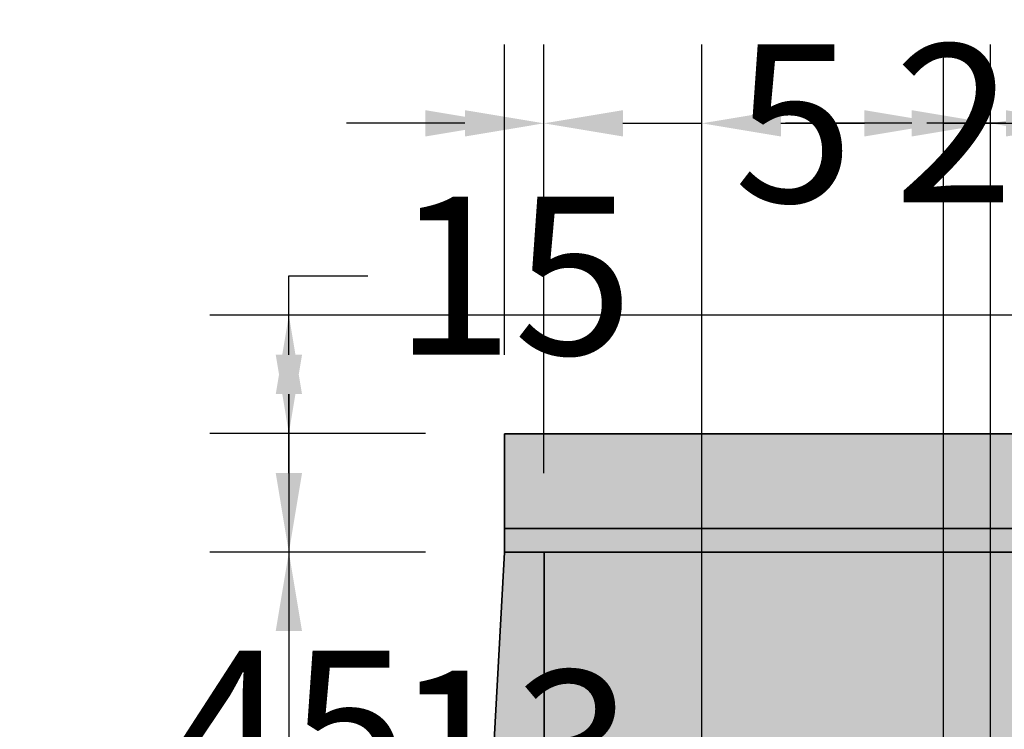
# Model space of a CAD drawing. Units: millimetres. Extents: x 130 to 1021, y 147 to 699.
# Tile 18 of 40: x 241 to 366, y 610 to 699. Entities that reach past the tile are written whole.
import ezdxf

# ---------------------------------------------------------------- set-up
doc = ezdxf.new("R2010")
doc.units = ezdxf.units.MM
doc.header["$MEASUREMENT"] = 0
for name, color, linetype, lineweight in [('A-ANNO-DIMS', 2, 'Continuous', 18), ('A-ELEV', 7, 'Continuous', 35), ('A-ELEV-PATT', 9, 'Continuous', 13)]:
    doc.layers.add(name, color=color, linetype=linetype, lineweight=lineweight)
doc.styles.get("Standard").update_dxf_attribs({"font": 'arial.ttf'})
doc.dimstyles.get("Standard").update_dxf_attribs({"dimtxt": 20, "dimasz": 10, "dimexe": 10, "dimexo": 10, "dimgap": 5, "dimtad": 0, "dimtih": 1, "dimtoh": 1, "dimdec": 0, "dimzin": 0, "dimdsep": 46, "dimtxsty": 'Standard', "dimcen": 5, "dimadec": 0, "dimazin": 0, "dimtfac": 1, "dimtdec": 0, "dimtofl": 0, "dimtmove": 0, "dimatfit": 3, "dimfxl": 1, "dimtolj": 1, "dimtzin": 0, "dimarcsym": 0})

# ---------------------------------------------------------------- blocks, each defined once
blk = doc.blocks.new('*D11')
at = {"layer": 'A-ANNO-DIMS', "color": 0, "lineweight": -2, "transparency": 16777216}
for p, q in [((737.37, 648.7), (737.37, 149.74)), ((299.37, 566.95), (299.37, 149.74)), ((309.37, 159.74), (490.86, 159.74)), ((727.37, 159.74), (545.89, 159.74))]:
    blk.add_line(p, q, dxfattribs=at)
at = {"layer": 'A-ANNO-DIMS', "color": 0, "transparency": 16777216}
for points in [[(309.37, 161.41), (309.37, 158.07), (299.37, 159.74)], [(727.37, 161.41), (727.37, 158.07), (737.37, 159.74)]]:
    blk.add_solid(points, dxfattribs=at)
at = {"layer": 'Defpoints', "color": 0, "transparency": 16777216}
for p in [(737.37, 658.7), (299.37, 576.95), (737.37, 159.74)]:
    blk.add_point(p, dxfattribs=at)
at = {"layer": 'A-ANNO-DIMS', "color": 0, "transparency": 16777216, "insert": (518.37, 159.74), "char_height": 20, "attachment_point": 5}
blk.add_mtext('\\A1;438', dxfattribs=at)
blk = doc.blocks.new('*D12')
at = {"layer": 'A-ANNO-DIMS', "color": 0, "lineweight": -2, "transparency": 16777216}
for p, q in [((477.37, 661.95), (265.07, 661.95)), ((275.07, 651.95), (275.07, 438.2)), ((275.07, 194.04), (275.07, 407.78)), ((357.16, 184.04), (265.07, 184.04))]:
    blk.add_line(p, q, dxfattribs=at)
at = {"layer": 'A-ANNO-DIMS', "color": 0, "transparency": 16777216}
for points in [[(273.41, 651.95), (276.74, 651.95), (275.07, 661.95)], [(273.41, 194.04), (276.74, 194.04), (275.07, 184.04)]]:
    blk.add_solid(points, dxfattribs=at)
at = {"layer": 'Defpoints', "color": 0, "transparency": 16777216}
for p in [(275.07, 661.95), (487.37, 661.95), (367.16, 184.04)]:
    blk.add_point(p, dxfattribs=at)
at = {"layer": 'A-ANNO-DIMS', "color": 0, "transparency": 16777216, "insert": (275.07, 422.99), "char_height": 20, "attachment_point": 5}
blk.add_mtext('\\A1;477.9', dxfattribs=at)
blk = doc.blocks.new('*D13')
at = {"layer": 'A-ANNO-DIMS', "color": 0, "lineweight": -2, "transparency": 16777216}
for p, q in [((302.37, 656.95), (302.37, 696.25)), ((307.37, 641.95), (307.37, 696.25)), ((292.37, 686.25), (282.37, 686.25)), ((317.37, 686.25), (327.37, 686.25))]:
    blk.add_line(p, q, dxfattribs=at)
at = {"layer": 'A-ANNO-DIMS', "color": 0, "transparency": 16777216}
for points in [[(292.37, 687.91), (292.37, 684.58), (302.37, 686.25)], [(317.37, 687.91), (317.37, 684.58), (307.37, 686.25)]]:
    blk.add_solid(points, dxfattribs=at)
at = {"layer": 'Defpoints', "color": 0, "transparency": 16777216}
for p in [(307.37, 686.25), (302.37, 646.95), (307.37, 631.95)]:
    blk.add_point(p, dxfattribs=at)
at = {"layer": 'A-ANNO-DIMS', "color": 0, "transparency": 16777216, "insert": (339, 686.25), "char_height": 20, "attachment_point": 5}
blk.add_mtext('\\A1;5', dxfattribs=at)
blk = doc.blocks.new('*D14')
at = {"layer": 'A-ANNO-DIMS', "color": 0, "lineweight": -2, "transparency": 16777216}
for p, q in [((307.37, 641.95), (307.37, 696.25)), ((327.37, 579.88), (327.37, 696.25)), ((297.37, 686.25), (287.37, 686.25)), ((337.37, 686.25), (347.37, 686.25))]:
    blk.add_line(p, q, dxfattribs=at)
at = {"layer": 'A-ANNO-DIMS', "color": 0, "transparency": 16777216}
for points in [[(297.37, 687.91), (297.37, 684.58), (307.37, 686.25)], [(337.37, 687.91), (337.37, 684.58), (327.37, 686.25)]]:
    blk.add_solid(points, dxfattribs=at)
at = {"layer": 'Defpoints', "color": 0, "transparency": 16777216}
for p in [(327.37, 686.25), (307.37, 631.95), (327.37, 569.88)]:
    blk.add_point(p, dxfattribs=at)
at = {"layer": 'A-ANNO-DIMS', "color": 0, "transparency": 16777216, "insert": (366.83, 686.25), "char_height": 20, "attachment_point": 5}
blk.add_mtext('\\A1;20', dxfattribs=at)
blk = doc.blocks.new('*D15')
at = {"layer": 'A-ANNO-DIMS', "color": 0, "lineweight": -2, "transparency": 16777216}
for p, q in [((327.37, 579.88), (327.37, 696.25)), ((357.94, 411.95), (357.94, 696.25)), ((337.37, 686.25), (347.94, 686.25)), ((357.94, 686.25), (367.94, 686.25))]:
    blk.add_line(p, q, dxfattribs=at)
at = {"layer": 'A-ANNO-DIMS', "color": 0, "transparency": 16777216}
for points in [[(337.37, 687.91), (337.37, 684.58), (327.37, 686.25)], [(347.94, 687.91), (347.94, 684.58), (357.94, 686.25)]]:
    blk.add_solid(points, dxfattribs=at)
at = {"layer": 'Defpoints', "color": 0, "transparency": 16777216}
for p in [(357.94, 686.25), (327.37, 569.88), (357.94, 401.95)]:
    blk.add_point(p, dxfattribs=at)
at = {"layer": 'A-ANNO-DIMS', "color": 0, "transparency": 16777216, "insert": (406.68, 686.25), "char_height": 20, "attachment_point": 5}
blk.add_mtext('\\A1;30.57', dxfattribs=at)
blk = doc.blocks.new('*D16')
at = {"layer": 'A-ANNO-DIMS', "color": 0, "lineweight": -2, "transparency": 16777216}
for p, q in [((357.94, 411.95), (357.94, 696.25)), ((363.92, 579.88), (363.92, 696.25)), ((347.94, 686.25), (337.94, 686.25)), ((373.92, 686.25), (383.92, 686.25))]:
    blk.add_line(p, q, dxfattribs=at)
at = {"layer": 'A-ANNO-DIMS', "color": 0, "transparency": 16777216}
for points in [[(347.94, 687.91), (347.94, 684.58), (357.94, 686.25)], [(373.92, 687.91), (373.92, 684.58), (363.92, 686.25)]]:
    blk.add_solid(points, dxfattribs=at)
at = {"layer": 'Defpoints', "color": 0, "transparency": 16777216}
for p in [(363.92, 686.25), (363.92, 569.88), (357.94, 401.95)]:
    blk.add_point(p, dxfattribs=at)
at = {"layer": 'A-ANNO-DIMS', "color": 0, "transparency": 16777216, "insert": (420.74, 686.25), "char_height": 20, "attachment_point": 5}
blk.add_mtext('\\A1;5.981', dxfattribs=at)
blk = doc.blocks.new('*D17')
at = {"layer": 'A-ANNO-DIMS', "color": 0, "lineweight": -2, "transparency": 16777216}
for p, q in [((363.92, 579.88), (363.92, 696.25)), ((375.85, 490.22), (375.85, 696.25)), ((353.92, 686.25), (343.92, 686.25)), ((385.85, 686.25), (395.85, 686.25))]:
    blk.add_line(p, q, dxfattribs=at)
at = {"layer": 'A-ANNO-DIMS', "color": 0, "transparency": 16777216}
for points in [[(353.92, 687.91), (353.92, 684.58), (363.92, 686.25)], [(385.85, 687.91), (385.85, 684.58), (375.85, 686.25)]]:
    blk.add_solid(points, dxfattribs=at)
at = {"layer": 'Defpoints', "color": 0, "transparency": 16777216}
for p in [(375.85, 686.25), (363.92, 569.88), (375.85, 480.22)]:
    blk.add_point(p, dxfattribs=at)
at = {"layer": 'A-ANNO-DIMS', "color": 0, "transparency": 16777216, "insert": (441.44, 686.25), "char_height": 20, "attachment_point": 5}
blk.add_mtext('\\A1;11.928', dxfattribs=at)
blk = doc.blocks.new('*D18')
at = {"layer": 'A-ANNO-DIMS', "color": 0, "lineweight": -2, "transparency": 16777216}
for p, q in [((375.85, 490.22), (375.85, 696.25)), ((382.37, 388.95), (382.37, 696.25)), ((365.85, 686.25), (355.85, 686.25)), ((392.37, 686.25), (402.37, 686.25))]:
    blk.add_line(p, q, dxfattribs=at)
at = {"layer": 'A-ANNO-DIMS', "color": 0, "transparency": 16777216}
for points in [[(365.85, 687.91), (365.85, 684.58), (375.85, 686.25)], [(392.37, 687.91), (392.37, 684.58), (382.37, 686.25)]]:
    blk.add_solid(points, dxfattribs=at)
at = {"layer": 'Defpoints', "color": 0, "transparency": 16777216}
for p in [(382.37, 686.25), (375.85, 480.22), (382.37, 378.95)]:
    blk.add_point(p, dxfattribs=at)
at = {"layer": 'A-ANNO-DIMS', "color": 0, "transparency": 16777216, "insert": (441.13, 686.25), "char_height": 20, "attachment_point": 5}
blk.add_mtext('\\A1;6.524', dxfattribs=at)
blk = doc.blocks.new('*D46')
at = {"layer": 'A-ANNO-DIMS', "color": 0, "lineweight": -2, "transparency": 16777216}
for p, q in [((275.07, 596.95), (275.07, 606.95)), ((275.07, 606.95), (285.07, 606.95)), ((292.37, 586.95), (265.07, 586.95)), ((292.37, 573.95), (265.07, 573.95)), ((275.07, 563.95), (275.07, 553.95))]:
    blk.add_line(p, q, dxfattribs=at)
at = {"layer": 'A-ANNO-DIMS', "color": 0, "transparency": 16777216}
for points in [[(273.41, 596.95), (276.74, 596.95), (275.07, 586.95)], [(273.41, 563.95), (276.74, 563.95), (275.07, 573.95)]]:
    blk.add_solid(points, dxfattribs=at)
at = {"layer": 'Defpoints', "color": 0, "transparency": 16777216}
for p in [(275.07, 586.95), (302.37, 586.95), (302.37, 573.95)]:
    blk.add_point(p, dxfattribs=at)
at = {"layer": 'A-ANNO-DIMS', "color": 0, "transparency": 16777216, "insert": (303.46, 606.95), "char_height": 20, "attachment_point": 5}
blk.add_mtext('\\A1;13', dxfattribs=at)
blk = doc.blocks.new('*D47')
at = {"layer": 'A-ANNO-DIMS', "color": 0, "lineweight": -2, "transparency": 16777216}
for p, q in [((275.07, 641.95), (275.07, 651.95)), ((292.37, 631.95), (265.07, 631.95)), ((292.37, 586.95), (265.07, 586.95)), ((275.07, 576.95), (275.07, 566.95))]:
    blk.add_line(p, q, dxfattribs=at)
at = {"layer": 'A-ANNO-DIMS', "color": 0, "transparency": 16777216}
for points in [[(273.41, 641.95), (276.74, 641.95), (275.07, 631.95)], [(273.41, 576.95), (276.74, 576.95), (275.07, 586.95)]]:
    blk.add_solid(points, dxfattribs=at)
at = {"layer": 'Defpoints', "color": 0, "transparency": 16777216}
for p in [(275.07, 631.95), (302.37, 631.95), (302.37, 586.95)]:
    blk.add_point(p, dxfattribs=at)
at = {"layer": 'A-ANNO-DIMS', "color": 0, "transparency": 16777216, "insert": (275.07, 609.45), "char_height": 20, "attachment_point": 5}
blk.add_mtext('\\A1;45', dxfattribs=at)
blk = doc.blocks.new('*D48')
at = {"layer": 'A-ANNO-DIMS', "color": 0, "lineweight": -2, "transparency": 16777216}
for p, q in [((275.07, 656.95), (275.07, 666.95)), ((275.07, 666.95), (285.07, 666.95)), ((292.37, 646.95), (265.07, 646.95)), ((292.37, 631.95), (265.07, 631.95)), ((275.07, 621.95), (275.07, 611.95))]:
    blk.add_line(p, q, dxfattribs=at)
at = {"layer": 'A-ANNO-DIMS', "color": 0, "transparency": 16777216}
for points in [[(273.41, 656.95), (276.74, 656.95), (275.07, 646.95)], [(273.41, 621.95), (276.74, 621.95), (275.07, 631.95)]]:
    blk.add_solid(points, dxfattribs=at)
at = {"layer": 'Defpoints', "color": 0, "transparency": 16777216}
for p in [(275.07, 646.95), (302.37, 646.95), (302.37, 631.95)]:
    blk.add_point(p, dxfattribs=at)
at = {"layer": 'A-ANNO-DIMS', "color": 0, "transparency": 16777216, "insert": (303.53, 666.95), "char_height": 20, "attachment_point": 5}
blk.add_mtext('\\A1;15', dxfattribs=at)

msp = doc.modelspace()

# ---------------------------------------------------------------- hatches: boundary and pattern name
at = {"layer": 'A-ELEV-PATT'}
h = msp.add_hatch(color=256, dxfattribs=at)
h.dxf.hatch_style = 1
h.paths.add_polyline_path([(737.3738, 658.6988, 0.01359606), (632.4019, 661.9473), (607.3738, 661.9473), (487.3738, 661.9473), (487.3738, 649.9473), (607.3738, 649.9473), (632.3794, 649.9473, -0.01368411), (737.3738, 646.6784)])
h.paths.add_polyline_path([(732.3738, 643.9599, 0.01305286), (632.3738, 646.9473), (607.3738, 646.9473), (487.3738, 646.9473), (487.3738, 596.9473), (632.3738, 596.9473, -0.01305286), (732.3738, 593.9599)])
h.paths.add_polyline_path([(737.3738, 593.6732, 0.01370629), (632.3738, 596.9473), (487.3738, 596.9473), (487.3738, 586.9473), (632.355, 586.9473, -0.01378075), (737.3738, 583.6559)])
h.paths.add_polyline_path([(447.3738, 646.9473), (307.3738, 646.9473), (302.3738, 646.9473), (302.3738, 634.9473), (447.3738, 634.9473)])
h.paths.add_polyline_path([(447.3738, 631.9473), (307.3738, 631.9473), (307.3738, 586.9473), (447.3738, 586.9473)])
h.paths.add_polyline_path([(447.3738, 586.9473), (307.3738, 586.9473), (302.3738, 586.9473), (302.3738, 576.9473), (447.3738, 576.9473)])
h.paths.add_polyline_path([(447.3738, 573.9473), (367.3738, 573.9473), (367.3738, 539.9473), (447.3738, 539.9473)])
h.paths.add_polyline_path([(447.3738, 537.9473), (367.3738, 537.9473), (367.3738, 507.9473), (400.392, 507.4253, -0.00172798), (401.3281, 507.6451, -0.52200255), (425.6117, 511.0391, -0.03918489), (447.3738, 510.4359), (447.3738, 510.7883)])
h.paths.add_polyline_path([(394.7238, 505.9473), (367.3738, 505.9473), (367.3738, 476.9473, -0.0146512), (375.8501, 480.2159), (376.1506, 499.2266, -0.03554194)])
h.paths.add_polyline_path([(632.3738, 583.9473), (552.3738, 583.9473), (552.3738, 550.9473), (632.3738, 550.9473)])
h.paths.add_polyline_path([(632.3738, 548.9473), (552.3738, 548.9473), (552.3738, 515.9473), (632.3738, 515.9473)])
h.paths.add_polyline_path([(632.3738, 513.9473), (552.3738, 513.9473), (552.3738, 476.9473), (632.3738, 476.9473)])
h.paths.add_polyline_path([(737.3738, 473.6903, 0.01363261), (632.3926, 476.9473), (552.3738, 476.9473), (487.3738, 476.9473), (487.3738, 466.9473), (632.3738, 466.9473, -0.01370629), (737.3738, 463.6732)])
h.paths.add_polyline_path([(732.3738, 460.9552, 0.01307409), (632.3681, 463.9473), (487.3738, 463.9473), (487.3738, 407.735, -0.00322862), (489.3544, 406.9473), (632.3926, 406.9473, -0.01298259), (732.3738, 403.9755)])
h.paths.add_polyline_path([(487.3738, 463.9473, 0.20132998), (367.3738, 463.9473), (367.3738, 407.735, -0.18820307), (487.3738, 407.735)])
h.paths.add_polyline_path([(367.3738, 476.9473), (367.3738, 466.9473, -0.20133085), (487.3738, 466.9473), (487.3738, 476.9473, 0.20132998)])
h.paths.add_polyline_path([(367.3738, 463.9473), (307.3738, 463.9473), (307.3738, 401.9473), (357.9413, 401.9473), (367.3738, 407.735)])
h.paths.add_polyline_path([(367.3738, 476.9473), (302.3738, 476.9473), (302.3738, 466.9473), (367.3738, 466.9473)])
h.paths.add_polyline_path([(632.8184, 366.9453), (552.3738, 366.9453), (552.3738, 393.9473), (632.8184, 393.9473)])
h.paths.add_polyline_path([(632.8184, 357.2114), (632.8184, 363.9453), (552.3738, 363.9453), (552.3738, 357.2114), (552.3738, 336.9453), (632.8184, 336.9453)])
h.paths.add_polyline_path([(632.8184, 333.9453), (552.3738, 333.9453), (552.3738, 306.9453), (632.8184, 306.9453)])
h.paths.add_polyline_path([(632.8184, 303.9453), (552.3738, 303.9453), (552.3738, 273.9473), (632.355, 273.9473, 0.00006077), (632.8184, 273.9491)])
h.paths.add_polyline_path([(737.3738, 403.6903, 0.01363261), (632.3926, 406.9473), (489.3544, 406.9473, 0.19154808), (367.3738, 407.735), (367.3738, 396.9473, -0.20133085), (487.3738, 396.9473), (632.3738, 396.9473, -0.01370629), (737.3738, 393.6732)])
h.paths.add_polyline_path([(357.9413, 401.9473), (307.3738, 401.9473), (307.3738, 391.9473), (357.9413, 391.9473)])
h.paths.add_polyline_path([(357.9413, 357.2114), (357.9413, 388.9473), (307.3738, 388.9473), (307.3738, 357.2114), (307.3738, 273.9473), (357.9413, 273.9473)])
h.paths.add_polyline_path([(732.3738, 263.93, -0.0130317), (632.3794, 260.9473), (466.7667, 260.9473), (466.7667, 240.9473), (469.8406, 236.978), (469.8406, 221.978), (472.9145, 218.0087), (472.9145, 213.9473), (607.3738, 213.9473), (732.3738, 213.9473)])
h.paths.add_polyline_path([(732.3738, 290.889), (722.479, 290.889), (722.479, 301.889), (732.3738, 301.889), (732.3738, 305.889), (722.479, 305.889), (722.479, 316.889), (732.3738, 316.889), (732.3738, 320.889), (722.479, 320.889), (722.479, 331.889), (732.3738, 331.889), (732.3738, 335.889), (722.479, 335.889), (722.479, 346.889), (732.3738, 346.889), (732.3738, 350.889), (722.479, 350.889), (722.479, 361.889), (732.3738, 361.889), (732.3738, 365.889), (722.479, 365.889), (722.479, 376.889), (732.3738, 376.889), (732.3738, 380.889), (722.479, 380.889), (722.479, 391.4848, 0.00052326), (718.479, 391.6843), (718.479, 380.889), (707.479, 380.889), (707.479, 392.1896, 0.00052307), (703.479, 392.3576), (703.479, 380.889), (692.479, 380.889), (692.479, 392.7765, 0.00052292), (688.479, 392.9131), (688.479, 380.889), (677.479, 380.889), (677.479, 393.2456, 0.00052279), (673.479, 393.3508), (673.479, 380.889), (662.479, 380.889), (662.479, 393.597, 0.0005227), (658.479, 393.6709), (658.479, 380.889), (647.479, 380.889), (647.479, 393.8308, 0.00052264), (643.479, 393.8732), (643.479, 380.889), (632.8184, 380.889), (632.8184, 376.889), (643.479, 376.889), (643.479, 365.889), (632.8184, 365.889), (632.8184, 361.889), (643.479, 361.889), (643.479, 350.889), (632.8184, 350.889), (632.8184, 346.889), (643.479, 346.889), (643.479, 335.889), (632.8184, 335.889), (632.8184, 331.889), (643.479, 331.889), (643.479, 320.889), (632.8184, 320.889), (632.8184, 316.889), (643.479, 316.889), (643.479, 305.889), (632.8184, 305.889), (632.8184, 301.889), (643.479, 301.889), (643.479, 290.889), (632.8184, 290.889), (632.8184, 286.889), (643.479, 286.889), (643.479, 274.0217, 0.00052456), (647.479, 274.0643), (647.479, 286.889), (658.479, 286.889), (658.479, 274.2248, 0.00052462), (662.479, 274.2989), (662.479, 286.889), (673.479, 286.889), (673.479, 274.546, 0.00052471), (677.479, 274.6516), (677.479, 286.889), (688.479, 286.889), (688.479, 274.9853, 0.00052484), (692.479, 275.1224), (692.479, 286.889), (703.479, 286.889), (703.479, 275.5429, 0.000525), (707.479, 275.7115), (707.479, 286.889), (718.479, 286.889), (718.479, 276.2187, 0.00052519), (722.479, 276.4189), (722.479, 286.889), (732.3738, 286.889)])
h.paths.add_polyline_path([(718.479, 290.889), (707.479, 290.889), (707.479, 301.889), (718.479, 301.889)], flags=16)
h.paths.add_polyline_path([(703.479, 290.889), (692.479, 290.889), (692.479, 301.889), (703.479, 301.889)], flags=16)
h.paths.add_polyline_path([(718.479, 305.889), (707.479, 305.889), (707.479, 316.889), (718.479, 316.889)], flags=16)
h.paths.add_polyline_path([(703.479, 305.889), (692.479, 305.889), (692.479, 316.889), (703.479, 316.889)], flags=16)
h.paths.add_polyline_path([(688.479, 290.889), (677.479, 290.889), (677.479, 301.889), (688.479, 301.889)], flags=16)
h.paths.add_polyline_path([(718.479, 320.889), (707.479, 320.889), (707.479, 331.889), (718.479, 331.889)], flags=16)
h.paths.add_polyline_path([(688.479, 305.889), (677.479, 305.889), (677.479, 316.889), (688.479, 316.889)], flags=16)
h.paths.add_polyline_path([(703.479, 320.889), (692.479, 320.889), (692.479, 331.889), (703.479, 331.889)], flags=16)
h.paths.add_polyline_path([(688.479, 320.889), (677.479, 320.889), (677.479, 331.889), (688.479, 331.889)], flags=16)
h.paths.add_polyline_path([(673.479, 290.889), (662.479, 290.889), (662.479, 301.889), (673.479, 301.889)], flags=16)
h.paths.add_polyline_path([(718.479, 335.889), (707.479, 335.889), (707.479, 346.889), (718.479, 346.889)], flags=16)
h.paths.add_polyline_path([(673.479, 305.889), (662.479, 305.889), (662.479, 316.889), (673.479, 316.889)], flags=16)
h.paths.add_polyline_path([(703.479, 335.889), (692.479, 335.889), (692.479, 346.889), (703.479, 346.889)], flags=16)
h.paths.add_polyline_path([(673.479, 320.889), (662.479, 320.889), (662.479, 331.889), (673.479, 331.889)], flags=16)
h.paths.add_polyline_path([(688.479, 335.889), (677.479, 335.889), (677.479, 346.889), (688.479, 346.889)], flags=16)
h.paths.add_polyline_path([(658.479, 290.889), (647.479, 290.889), (647.479, 301.889), (658.479, 301.889)], flags=16)
h.paths.add_polyline_path([(718.479, 350.889), (707.479, 350.889), (707.479, 361.889), (718.479, 361.889)], flags=16)
h.paths.add_polyline_path([(658.479, 305.889), (647.479, 305.889), (647.479, 316.889), (658.479, 316.889)], flags=16)
h.paths.add_polyline_path([(703.479, 350.889), (692.479, 350.889), (692.479, 361.889), (703.479, 361.889)], flags=16)
h.paths.add_polyline_path([(673.479, 335.889), (662.479, 335.889), (662.479, 346.889), (673.479, 346.889)], flags=16)
h.paths.add_polyline_path([(658.479, 320.889), (647.479, 320.889), (647.479, 331.889), (658.479, 331.889)], flags=16)
h.paths.add_polyline_path([(688.479, 350.889), (677.479, 350.889), (677.479, 361.889), (688.479, 361.889)], flags=16)
h.paths.add_polyline_path([(718.479, 365.889), (707.479, 365.889), (707.479, 376.889), (718.479, 376.889)], flags=16)
h.paths.add_polyline_path([(658.479, 335.889), (647.479, 335.889), (647.479, 346.889), (658.479, 346.889)], flags=16)
h.paths.add_polyline_path([(673.479, 350.889), (662.479, 350.889), (662.479, 361.889), (673.479, 361.889)], flags=16)
h.paths.add_polyline_path([(703.479, 365.889), (692.479, 365.889), (692.479, 376.889), (703.479, 376.889)], flags=16)
h.paths.add_polyline_path([(688.479, 365.889), (677.479, 365.889), (677.479, 376.889), (688.479, 376.889)], flags=16)
h.paths.add_polyline_path([(658.479, 350.889), (647.479, 350.889), (647.479, 361.889), (658.479, 361.889)], flags=16)
h.paths.add_polyline_path([(673.479, 365.889), (662.479, 365.889), (662.479, 376.889), (673.479, 376.889)], flags=16)
h.paths.add_polyline_path([(658.479, 365.889), (647.479, 365.889), (647.479, 376.889), (658.479, 376.889)], flags=16)
h.paths.add_polyline_path([(732.3738, 503.9786), (722.3392, 503.9786), (722.3392, 514.9786), (732.3738, 514.9786), (732.3738, 518.9786), (722.3392, 518.9786), (722.3392, 529.9786), (732.3738, 529.9786), (732.3738, 533.9786), (722.3392, 533.9786), (722.3392, 544.9786), (732.3738, 544.9786), (732.3738, 546.9473), (732.3738, 548.9786), (722.3392, 548.9786), (722.3392, 559.9786), (732.3738, 559.9786), (732.3738, 563.9786), (722.3392, 563.9786), (722.3392, 574.9786), (732.3738, 574.9786), (732.3738, 578.9786), (722.3392, 578.9786), (722.3392, 581.4789, 0.00052601), (718.3392, 581.6791), (718.3392, 578.9786), (707.3392, 578.9786), (707.3392, 582.1863, 0.00052582), (703.3392, 582.355), (703.3392, 578.9786), (692.3392, 578.9786), (692.3392, 582.7752, 0.00052566), (688.3392, 582.9123), (688.3392, 578.9786), (677.3392, 578.9786), (677.3392, 583.2457, 0.00052554), (673.3392, 583.3512), (673.3392, 578.9786), (662.3392, 578.9786), (662.3392, 583.5978, 0.00052545), (658.3392, 583.6718), (658.3392, 578.9786), (647.3392, 578.9786), (647.3392, 583.8317, 0.00052539), (643.3392, 583.8741), (643.3392, 578.9786), (632.3738, 578.9786), (632.3738, 574.9786), (643.3392, 574.9786), (643.3392, 563.9786), (632.3738, 563.9786), (632.3738, 559.9786), (643.3392, 559.9786), (643.3392, 548.9786), (632.3738, 548.9786), (632.3738, 544.9786), (643.3392, 544.9786), (643.3392, 533.9786), (632.3738, 533.9786), (632.3738, 529.9786), (643.3392, 529.9786), (643.3392, 518.9786), (632.3738, 518.9786), (632.3738, 515.9473), (632.3738, 514.9786), (643.3392, 514.9786), (643.3392, 503.9786), (632.3738, 503.9786), (632.3738, 499.9786), (643.3392, 499.9786), (643.3392, 488.9786), (632.3738, 488.9786), (632.3738, 484.9786), (643.3392, 484.9786), (643.3392, 476.8751, -0.00051911), (647.3392, 476.8332), (647.3392, 484.9786), (658.3392, 484.9786), (658.3392, 476.6752, -0.00051917), (662.3392, 476.6022), (662.3392, 484.9786), (673.3392, 484.9786), (673.3392, 476.3585, -0.00051926), (677.3392, 476.2543), (677.3392, 484.9786), (688.3392, 484.9786), (688.3392, 475.9248, -0.00051938), (692.3392, 475.7894), (692.3392, 484.9786), (703.3392, 484.9786), (703.3392, 475.3741, -0.00051953), (707.3392, 475.2075), (707.3392, 484.9786), (718.3392, 484.9786), (718.3392, 474.7064, -0.00051972), (722.3392, 474.5086), (722.3392, 484.9786), (732.3738, 484.9786), (732.3738, 488.9786), (722.3392, 488.9786), (722.3392, 499.9786), (732.3738, 499.9786)])
h.paths.add_polyline_path([(718.3392, 503.9786), (707.3392, 503.9786), (707.3392, 514.9786), (718.3392, 514.9786)], flags=16)
h.paths.add_polyline_path([(718.3392, 499.9786), (718.3392, 488.9786), (707.3392, 488.9786), (707.3392, 499.9786)], flags=16)
h.paths.add_polyline_path([(718.3392, 518.9786), (707.3392, 518.9786), (707.3392, 529.9786), (718.3392, 529.9786)], flags=16)
h.paths.add_polyline_path([(703.3392, 503.9786), (692.3392, 503.9786), (692.3392, 514.9786), (703.3392, 514.9786)], flags=16)
h.paths.add_polyline_path([(703.3392, 499.9786), (703.3392, 488.9786), (692.3392, 488.9786), (692.3392, 499.9786)], flags=16)
h.paths.add_polyline_path([(703.3392, 518.9786), (692.3392, 518.9786), (692.3392, 529.9786), (703.3392, 529.9786)], flags=16)
h.paths.add_polyline_path([(718.3392, 533.9786), (707.3392, 533.9786), (707.3392, 544.9786), (718.3392, 544.9786)], flags=16)
h.paths.add_polyline_path([(688.3392, 503.9786), (677.3392, 503.9786), (677.3392, 514.9786), (688.3392, 514.9786)], flags=16)
h.paths.add_polyline_path([(688.3392, 499.9786), (688.3392, 488.9786), (677.3392, 488.9786), (677.3392, 499.9786)], flags=16)
h.paths.add_polyline_path([(703.3392, 533.9786), (692.3392, 533.9786), (692.3392, 544.9786), (703.3392, 544.9786)], flags=16)
h.paths.add_polyline_path([(688.3392, 518.9786), (677.3392, 518.9786), (677.3392, 529.9786), (688.3392, 529.9786)], flags=16)
h.paths.add_polyline_path([(688.3392, 533.9786), (677.3392, 533.9786), (677.3392, 544.9786), (688.3392, 544.9786)], flags=16)
h.paths.add_polyline_path([(718.3392, 548.9786), (707.3392, 548.9786), (707.3392, 559.9786), (718.3392, 559.9786)], flags=16)
h.paths.add_polyline_path([(673.3392, 503.9786), (662.3392, 503.9786), (662.3392, 514.9786), (673.3392, 514.9786)], flags=16)
h.paths.add_polyline_path([(673.3392, 499.9786), (673.3392, 488.9786), (662.3392, 488.9786), (662.3392, 499.9786)], flags=16)
h.paths.add_polyline_path([(703.3392, 548.9786), (692.3392, 548.9786), (692.3392, 559.9786), (703.3392, 559.9786)], flags=16)
h.paths.add_polyline_path([(673.3392, 518.9786), (662.3392, 518.9786), (662.3392, 529.9786), (673.3392, 529.9786)], flags=16)
h.paths.add_polyline_path([(688.3392, 548.9786), (677.3392, 548.9786), (677.3392, 559.9786), (688.3392, 559.9786)], flags=16)
h.paths.add_polyline_path([(673.3392, 533.9786), (662.3392, 533.9786), (662.3392, 544.9786), (673.3392, 544.9786)], flags=16)
h.paths.add_polyline_path([(718.3392, 563.9786), (707.3392, 563.9786), (707.3392, 574.9786), (718.3392, 574.9786)], flags=16)
h.paths.add_polyline_path([(658.3392, 503.9786), (647.3392, 503.9786), (647.3392, 514.9786), (658.3392, 514.9786)], flags=16)
h.paths.add_polyline_path([(658.3392, 499.9786), (658.3392, 488.9786), (647.3392, 488.9786), (647.3392, 499.9786)], flags=16)
h.paths.add_polyline_path([(703.3392, 563.9786), (692.3392, 563.9786), (692.3392, 574.9786), (703.3392, 574.9786)], flags=16)
h.paths.add_polyline_path([(658.3392, 518.9786), (647.3392, 518.9786), (647.3392, 529.9786), (658.3392, 529.9786)], flags=16)
h.paths.add_polyline_path([(673.3392, 548.9786), (662.3392, 548.9786), (662.3392, 559.9786), (673.3392, 559.9786)], flags=16)
h.paths.add_polyline_path([(688.3392, 563.9786), (677.3392, 563.9786), (677.3392, 574.9786), (688.3392, 574.9786)], flags=16)
h.paths.add_polyline_path([(658.3392, 533.9786), (647.3392, 533.9786), (647.3392, 544.9786), (658.3392, 544.9786)], flags=16)
h.paths.add_polyline_path([(673.3392, 563.9786), (662.3392, 563.9786), (662.3392, 574.9786), (673.3392, 574.9786)], flags=16)
h.paths.add_polyline_path([(658.3392, 548.9786), (647.3392, 548.9786), (647.3392, 559.9786), (658.3392, 559.9786)], flags=16)
h.paths.add_polyline_path([(658.3392, 563.9786), (647.3392, 563.9786), (647.3392, 574.9786), (658.3392, 574.9786)], flags=16)
h = msp.add_hatch(color=256, dxfattribs=at)
h.dxf.hatch_style = 1
h.paths.add_polyline_path([(447.3738, 634.9473), (302.3738, 634.9473), (302.3738, 631.9473), (307.3738, 631.9473), (447.3738, 631.9473)])
h.paths.add_polyline_path([(487.3738, 646.9473), (487.3738, 649.9473), (447.3738, 634.9473), (447.3738, 631.9473)])
h.paths.add_polyline_path([(632.3794, 649.9473), (607.3738, 649.9473), (487.3738, 649.9473), (487.3738, 646.9473), (607.3738, 646.9473), (632.3738, 646.9473, -0.01370629), (737.3738, 643.6732), (737.3738, 646.6784, 0.01368411)])
h = msp.add_hatch(color=256, dxfattribs=at)
h.paths.add_polyline_path([(299.3738, 576.9473), (302.3738, 576.9473), (302.3738, 586.9473), (307.3738, 586.9473), (307.3738, 631.9473), (302.3738, 631.9473)])
h.paths.add_polyline_path([(304.0806, 532.6995), (307.3738, 532.6995), (307.3738, 573.9473)])

# ---------------------------------------------------------------- linework, layer by layer
at = {"layer": 'A-ELEV'}
for p, q in [((307.3738, 646.9473), (302.3738, 646.9473)), ((302.3738, 646.9473), (302.3738, 631.9473)), ((447.3738, 646.9473), (307.3738, 646.9473)), ((447.3738, 634.9473), (302.3738, 634.9473)), ((299.3738, 576.9473), (302.3738, 631.9473)), ((302.3738, 631.9473), (307.3738, 631.9473)), ((307.3738, 631.9473), (307.3738, 586.9473)), ((447.3738, 631.9473), (307.3738, 631.9473))]:
    msp.add_line(p, q, dxfattribs=at)

# ---------------------------------------------------------------- dimensions: what is measured, and where the dimension line sits
at = {"layer": 'A-ANNO-DIMS'}
for base, p1, p2, override, picture, middle in [((307.3738, 686.2473), (302.3738, 646.9473), (307.3738, 631.9473), {"dimdec": 0, "dimlfac": 1, "dimrnd": 0, "dimzin": 0, "dimdsep": 46, "dimlunit": 2}, '*D13', (339.0041, 686.2473)), ((327.3738, 686.2473), (307.3738, 631.9473), (327.3738, 569.884), {"dimdec": 0, "dimlfac": 1, "dimrnd": 0, "dimzin": 0, "dimdsep": 46, "dimlunit": 2}, '*D14', (366.8349, 686.2473)), ((357.9413, 686.2473), (327.3738, 569.884), (357.9413, 401.9473), {"dimdec": 2, "dimlfac": 1, "dimrnd": 0, "dimzin": 0, "dimdsep": 46, "dimlunit": 2}, '*D15', (406.6794, 686.2473)), ((363.922, 686.2473), (357.9413, 401.9473), (363.922, 569.884), {"dimdec": 3, "dimlfac": 1, "dimrnd": 0, "dimzin": 0, "dimdsep": 46, "dimlunit": 2}, '*D16', (420.7365, 686.2473)), ((375.8501, 686.2473), (363.922, 569.884), (375.8501, 480.2159), {"dimdec": 3, "dimlfac": 1, "dimrnd": 0, "dimzin": 0, "dimdsep": 46, "dimlunit": 2}, '*D17', (441.4435, 686.2473)), ((382.3738, 686.2473), (375.8501, 480.2159), (382.3738, 378.9473), {"dimdec": 3, "dimlfac": 1, "dimrnd": 0, "dimzin": 0, "dimdsep": 46, "dimlunit": 2}, '*D18', (441.1323, 686.2473)), ((737.3738, 159.7395), (299.3738, 576.9473), (737.3738, 658.6988), {"dimdec": 0, "dimlfac": 1, "dimrnd": 0, "dimzin": 0, "dimdsep": 46, "dimlunit": 2}, '*D11', (518.3738, 159.7395))]:
    dim = msp.add_linear_dim(base=base, p1=p1, p2=p2, dimstyle='Standard', override=override, dxfattribs=at)
    dim.commit()
    dim.dimension.update_dxf_attribs({"geometry": picture, "text_midpoint": middle})
for base, p1, p2, override, picture, middle in [((275.0738, 646.9473), (302.3738, 631.9473), (302.3738, 646.9473), {"dimdec": 0, "dimlfac": 1, "dimrnd": 0, "dimzin": 0, "dimdsep": 46, "dimlunit": 2}, '*D48', (303.5322, 666.9473)), ((275.0738, 661.9473), (367.163, 184.0395), (487.3738, 661.9473), {"dimdec": 1, "dimlfac": 1, "dimrnd": 0, "dimzin": 0, "dimdsep": 46, "dimlunit": 2}, '*D12', (275.0738, 422.9934)), ((275.0738, 631.9473), (302.3738, 586.9473), (302.3738, 631.9473), {"dimdec": 0, "dimlfac": 1, "dimrnd": 0, "dimzin": 0, "dimdsep": 46, "dimlunit": 2}, '*D47', (275.0738, 609.4473)), ((275.0738, 586.9473), (302.3738, 573.9473), (302.3738, 586.9473), {"dimdec": 0, "dimlfac": 1, "dimrnd": 0, "dimzin": 0, "dimdsep": 46, "dimlunit": 2}, '*D46', (303.4571, 606.9473))]:
    dim = msp.add_linear_dim(base=base, p1=p1, p2=p2, angle=90, dimstyle='Standard', override=override, dxfattribs=at)
    dim.commit()
    dim.dimension.update_dxf_attribs({"geometry": picture, "text_midpoint": middle})

doc.saveas('drawing.dxf')
